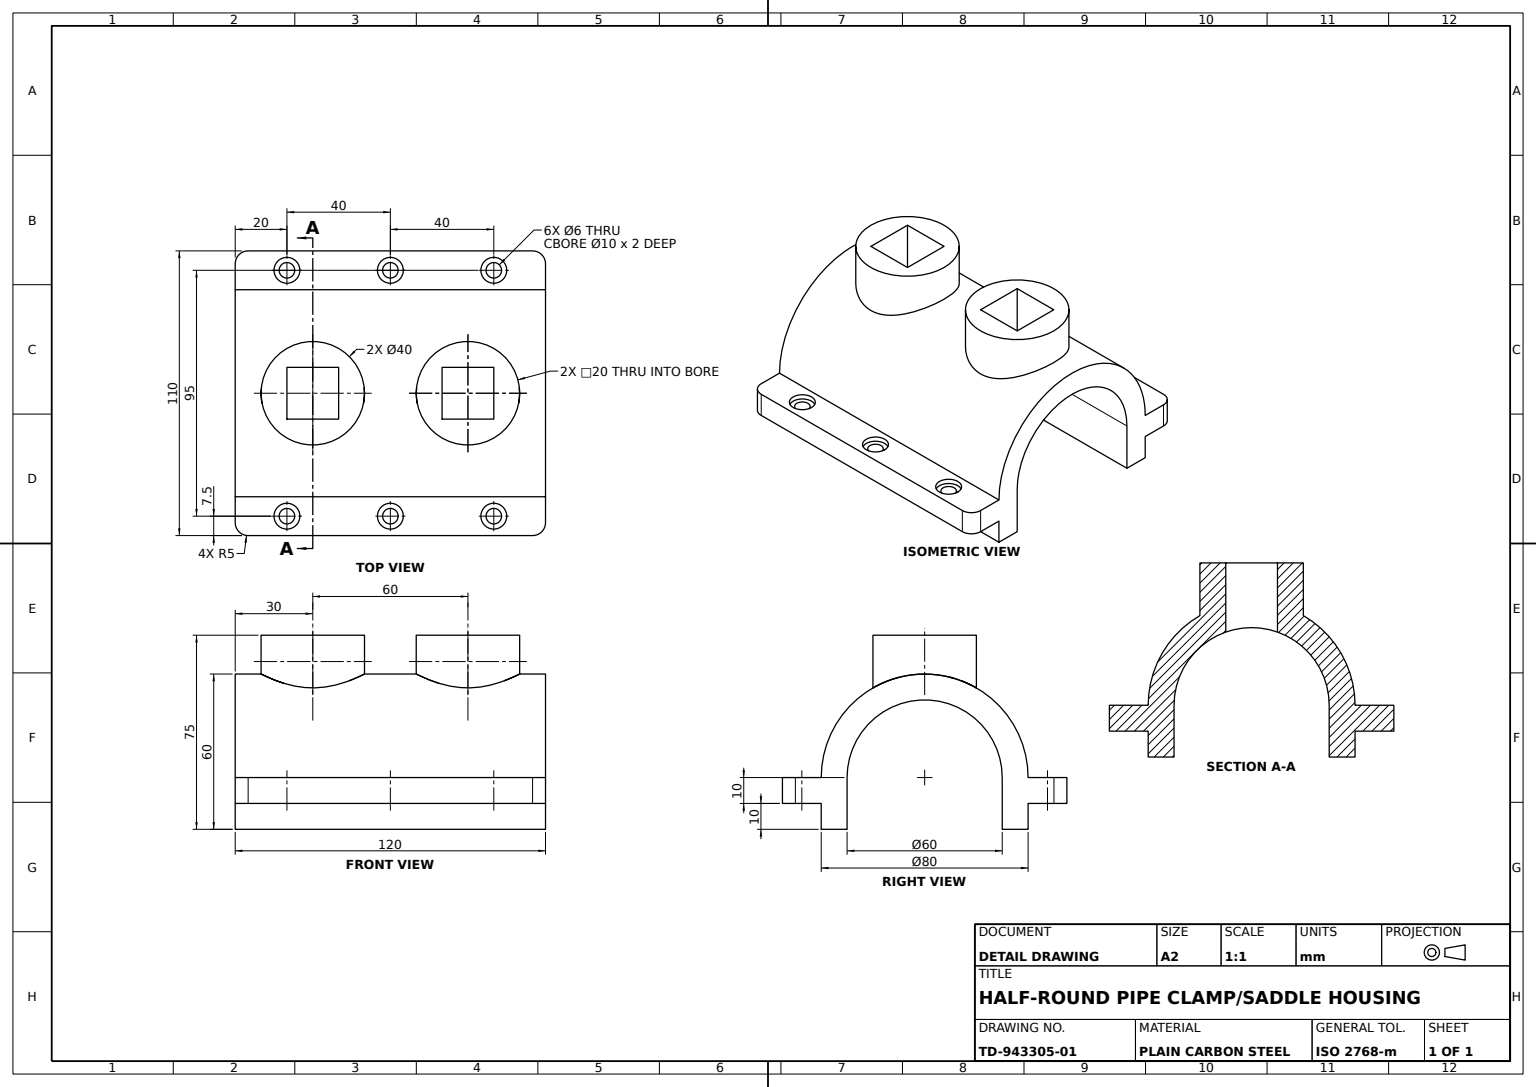
SolidWorks part; units mm, degrees
material "Plain Carbon Steel"
ref_plane "Front Plane" through (0, 0, 0) normal (0, 0, 1) x (1, 0, 0)
ref_plane "Top Plane" through (0, 0, 0) normal (0, 1, 0) x (1, 0, 0)
ref_plane "Right Plane" through (0, 0, 0) normal (1, 0, 0) x (0, 0, -1)
sketch "Saddle Profile Sketch" plane through (0, 0, 0) normal (0, 0, 1) x (1, 0, 0)
  line L0 (-40, 0) -> (-40, -20)
  line L1 (-40, -20) -> (-30, -20)
  line L2 (40, -20) -> (40, 0)
  line L3 (-30, 0) -> (-30, -20)
  line L4 (30, 0) -> (30, -20)
  line L5 (30, -20) -> (40, -20)
  arc A0 (40, 0) -> (-40, 0) centre (0, 0) ccw
  arc A1 (30, 0) -> (-30, 0) centre (0, 0) ccw
  dimension "D1" = 80
  dimension "D2" = 60
  dimension "D3" = 20
extrude "Saddle Body" add sketch "Saddle Profile Sketch" against normal blind 120
sketch "Flange Sketch" plane through (0, 0, 0) normal (0, 1, 0) x (1, 0, 0)
  line L0 (0, 0) -> (0, 18.828) construction
  line L1 (40, 120) -> (55, 120)
  line L2 (40, 120) -> (40, 0)
  line L3 (40, 0) -> (55, 0)
  line L4 (55, 120) -> (55, 0)
  line L5 (-40, 120) -> (-55, 120)
  line L6 (-40, 120) -> (-40, 0)
  line L7 (-40, 0) -> (-55, 0)
  line L8 (-55, 120) -> (-55, 0)
  point P13 (-47.5, 0)
  point P14 (47.5, 0)
  dimension "D1" = 95
  dimension "D2" = 7.5
  dimension "D3" = 120
extrude "Mounting Flange" add sketch "Flange Sketch" against normal blind 10
sketch "Flange Hole Positions" plane through (0, 0, 0) normal (0, 1, 0) x (1, 0, 0)
  line L0 (55, 120) -> (40, 120) construction
  line L1 (40, 0) -> (55, 0) construction
  line L2 (-55, 120) -> (-55, 0) construction
  line L3 (55, 0) -> (55, 120) construction
  circle A0 centre (47.5, 100) radius 5
  circle A1 centre (47.5, 60) radius 5
  circle A2 centre (47.5, 20) radius 5
  circle A3 centre (-47.5, 100) radius 5
  circle A4 centre (-47.5, 60) radius 5
  circle A5 centre (-47.5, 20) radius 5
  dimension "D1" = 10
  dimension "D2" = 20
  dimension "D3" = 20
  dimension "D4" = 60
  dimension "D5" = 7.5
  dimension "D6" = 7.5
hole_wizard "Counterbored Flange Holes Ø6" positions "Sketch4" profile "Sketch5" legacy
sketch "Sketch4" plane through (0, 0, 0) normal (0, 1, 0) x (1, 0, 0)
  point P0 (-47.5, 100)
  point P3 (-47.5, 60)
  point P6 (-47.5, 20)
  point P9 (47.5, 20)
  point P12 (47.5, 60)
  point P15 (47.5, 100)
sketch "Sketch5" plane through (-47.5, 0, -100) normal (1, 0, 0) x (0, 0, 1)
  line L0 (0, 0) -> (0, 11.8322)
  line L1 (0, 11.8322) -> (3, 11.8322)
  line L2 (3, 11.8322) -> (3, 2)
  line L3 (3, 2) -> (5, 2)
  line L4 (5, 2) -> (5, 0)
  line L5 (5, 0) -> (0, 0)
  line L6 (0, 110) -> (0, -10) construction
  dimension "Diameter" = 6
  dimension "Depth" = 12
  dimension "C-Bore Diameter" = 10
  dimension "C-Bore Depth" = 2
ref_plane "Boss Top Plane" through (0, 55, 0) normal (0, 1, 0) x (1, 0, 0)
sketch "Twin Boss Sketch" plane through (0, 55, 0) normal (0, 1, 0) x (1, 0, 0)
  line L0 (-47.5, 60) -> (-42.5, 60) construction
  circle A0 centre (0, 90) radius 20
  circle A1 centre (0, 30) radius 20
  circle A2 centre (-47.5, 60) radius 5 construction
  dimension "D1" = 40
  dimension "D2" = 30
  dimension "D3" = 30
extrude "Twin Bosses" add sketch "Twin Boss Sketch" against normal up to next
sketch "Square Socket Sketch" plane through (0, 55, 0) normal (0, 1, 0) x (1, 0, 0)
  line L1 (-10, 80) -> (10, 80)
  line L2 (-10, 80) -> (-10, 100)
  line L3 (-10, 100) -> (10, 100)
  line L4 (10, 80) -> (10, 100)
  line L5 (-10, 80) -> (10, 100) construction
  line L6 (-10, 100) -> (10, 80) construction
  line L7 (-10, 20) -> (10, 20)
  line L8 (-10, 20) -> (-10, 40)
  line L9 (-10, 40) -> (10, 40)
  line L10 (10, 20) -> (10, 40)
  line L11 (-10, 20) -> (10, 40) construction
  line L12 (-10, 40) -> (10, 20) construction
  point P0 (0, 90)
  point P5 (0, 30)
  dimension "D1" = 20
  dimension "D2" = 20
  dimension "D3" = 20
  dimension "D4" = 20
extrude "Square Sockets 20x20" cut sketch "Square Socket Sketch" against normal through all
fillet "Flange Fillet R5" radius 5 4 edges at (-55, -5, -120) (-55, -5, 0) (55, -5, -120) (55, -5, 0)
